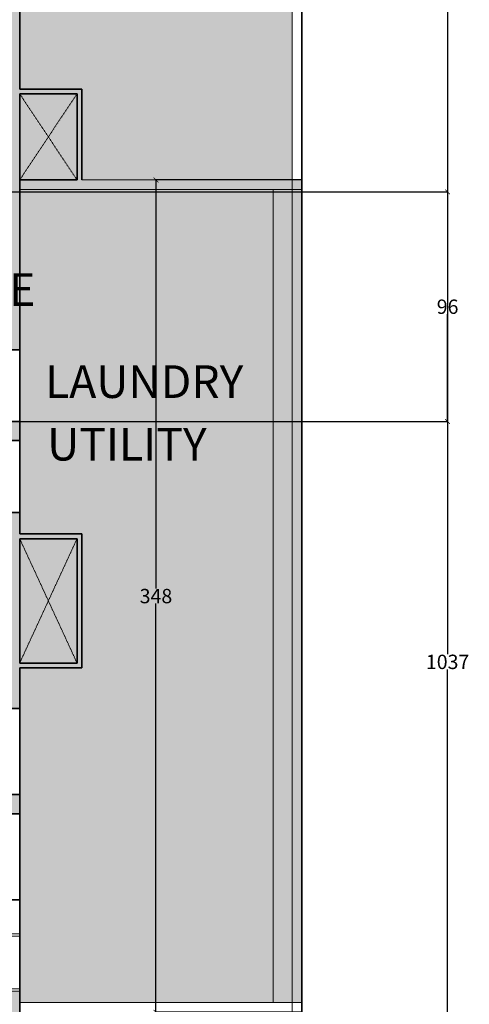
# Model space of a CAD drawing. Units: inches. Extents: x 1704 to 6393, y -157 to 1172.
# Tile 88 of 122: x 2605 to 2793, y 372 to 783. Entities that reach past the tile are written whole.
import ezdxf

# ---------------------------------------------------------------- set-up
doc = ezdxf.new("R2010")
doc.units = ezdxf.units.IN
doc.header["$MEASUREMENT"] = 0
doc.linetypes.add('HIDDEN', pattern=[0.375, 0.25, -0.125])
for name, color, linetype, lineweight in [('A-ANNO-DIMS', 7, 'Continuous', 13), ('A-AREA-IDEN', 7, 'Continuous', 18), ('A-FLOR-OPEN-HIDN', 8, 'HIDDEN', 13), ('A-WALL-PATT', 7, 'Continuous', 13), ('C-PROP', 7, 'Continuous', 35), ('L-HRDS', 8, 'Continuous', 18), ('L-PVMT-PATT', 8, 'Continuous', 13), ('WALLS', 7, 'Continuous', 35), ('WINDOWS', 2, 'Continuous', 18)]:
    doc.layers.add(name, color=color, linetype=linetype, lineweight=lineweight)
doc.layers.add('A-FLOR-PATT', color=7, linetype='Continuous', lineweight=13, true_color=0xf2f2f2)
doc.layers.add('L-HRDS-PATT', color=9, linetype='Continuous', lineweight=13, true_color=0xc5c1ba)
doc.styles.get("Standard").update_dxf_attribs({"font": 'arial.ttf'})
doc.dimstyles.get("Standard").update_dxf_attribs({"dimtxt": 6, "dimasz": 2, "dimexe": 0.18, "dimexo": 0.0625, "dimgap": 0.09, "dimtad": 0, "dimtih": 1, "dimtoh": 1, "dimdec": 1, "dimzin": 0, "dimdsep": 46, "dimlunit": 3, "dimtxsty": 'Standard', "dimblk": 'ARCHTICK', "dimcen": 0.09, "dimadec": 0, "dimazin": 0, "dimtfac": 1, "dimtdec": 1, "dimtofl": 0, "dimtmove": 0, "dimatfit": 3, "dimfxl": 1, "dimtolj": 1, "dimtzin": 0, "dimarcsym": 0})

# ---------------------------------------------------------------- blocks, each defined once
blk = doc.blocks.new('WIN-VENT-24')
for p, q in [((0, 0), (0, 24)), ((0, 24), (8, 24)), ((0, 23), (3.5, 23)), ((3.5, 23), (3.5, 1)), ((4.5, 23), (8, 23)), ((4.5, 23), (4.5, 1)), ((8, 24), (8, 0)), ((3.5, 1), (0, 1)), ((8, 1), (4.5, 1)), ((8, 0), (0, 0))]:
    blk.add_line(p, q)
blk = doc.blocks.new('_ArchTick')
at = {"color": 0, "linetype": 'ByBlock', "const_width": 0.15}
blk.add_lwpolyline([(-0.5, -0.5), (0.5, 0.5)], dxfattribs=at)
blk = doc.blocks.new('*D91')
at = {"layer": 'A-ANNO-DIMS', "color": 0, "lineweight": -2, "transparency": 16777216}
for p, q in [((2723.41, 1033.21), (2784.53, 1033.21)), ((2784.35, 1033.21), (2784.35, 517.87)), ((2784.35, -3.79), (2784.35, 511.56)), ((2723.41, -3.79), (2784.53, -3.79))]:
    blk.add_line(p, q, dxfattribs=at)
at = {"layer": 'Defpoints', "color": 0, "lineweight": -3, "transparency": 16777216}
for p in [(2723.35, 1033.21), (2784.35, 1033.21), (2723.35, -3.79)]:
    blk.add_point(p, dxfattribs=at)
at = {"layer": 'A-ANNO-DIMS', "color": 0, "lineweight": -2, "transparency": 16777216, "xscale": 2, "yscale": 2, "zscale": 2}
for p, rotation in [((2784.35, 1033.21), 90), ((2784.35, -3.79), 270)]:
    blk.add_blockref('_ArchTick', p, dxfattribs=dict(at, rotation=rotation))
at = {"layer": 'A-ANNO-DIMS', "color": 0, "transparency": 16777216, "insert": (2784.35, 514.71), "char_height": 6, "attachment_point": 5}
blk.add_mtext('\\A1;1037', dxfattribs=at)
blk = doc.blocks.new('*D97')
at = {"layer": 'A-ANNO-DIMS', "color": 0, "lineweight": -2, "transparency": 16777216}
for p, q in [((2723.29, 716.21), (2662.17, 716.21)), ((2662.35, 716.21), (2662.35, 545.37)), ((2662.35, 368.21), (2662.35, 539.06)), ((2723.29, 368.21), (2662.17, 368.21))]:
    blk.add_line(p, q, dxfattribs=at)
at = {"layer": 'Defpoints', "color": 0, "lineweight": -3, "transparency": 16777216}
for p in [(2662.35, 716.21), (2723.35, 716.21), (2723.35, 368.21)]:
    blk.add_point(p, dxfattribs=at)
at = {"layer": 'A-ANNO-DIMS', "color": 0, "lineweight": -2, "transparency": 16777216, "xscale": 2, "yscale": 2, "zscale": 2}
for p, rotation in [((2662.35, 716.21), 90), ((2662.35, 368.21), 270)]:
    blk.add_blockref('_ArchTick', p, dxfattribs=dict(at, rotation=rotation))
at = {"layer": 'A-ANNO-DIMS', "color": 0, "transparency": 16777216, "insert": (2662.35, 542.21), "char_height": 6, "attachment_point": 5}
blk.add_mtext('\\A1;348', dxfattribs=at)
blk = doc.blocks.new('*D101')
at = {"layer": 'A-ANNO-DIMS', "color": 0, "lineweight": -2, "transparency": 16777216}
for p, q in [((2547.41, 711.21), (2784.53, 711.21)), ((2784.35, 711.21), (2784.35, 666.37)), ((2784.35, 615.21), (2784.35, 660.06)), ((2547.41, 615.21), (2784.53, 615.21))]:
    blk.add_line(p, q, dxfattribs=at)
at = {"layer": 'Defpoints', "color": 0, "lineweight": -3, "transparency": 16777216}
for p in [(2547.35, 711.21), (2784.35, 711.21), (2547.35, 615.21)]:
    blk.add_point(p, dxfattribs=at)
at = {"layer": 'A-ANNO-DIMS', "color": 0, "lineweight": -2, "transparency": 16777216, "xscale": 2, "yscale": 2, "zscale": 2}
for p, rotation in [((2784.35, 711.21), 90), ((2784.35, 615.21), 270)]:
    blk.add_blockref('_ArchTick', p, dxfattribs=dict(at, rotation=rotation))
at = {"layer": 'A-ANNO-DIMS', "color": 0, "transparency": 16777216, "insert": (2784.35, 663.21), "char_height": 6, "attachment_point": 5}
blk.add_mtext('\\A1;96', dxfattribs=at)

msp = doc.modelspace()

# ---------------------------------------------------------------- hatches: boundary and pattern name
at = {"layer": 'A-FLOR-PATT'}
h = msp.add_hatch(color=256, dxfattribs=at)
h.dxf.hatch_style = 1
h.paths.add_polyline_path([(2629.349, 566.213), (2617.349, 540.213), (2629.349, 514.213)])
h.paths.add_polyline_path([(2629.349, 566.213), (2605.349, 566.213), (2617.349, 540.213)])
h.paths.add_polyline_path([(2605.349, 566.213), (2605.349, 514.213), (2617.349, 540.213)])
h.paths.add_polyline_path([(2617.349, 540.213), (2605.349, 514.213), (2629.349, 514.213)])
h.paths.add_polyline_path([(2617.349, 734.213), (2605.349, 716.213), (2629.349, 716.213)])
h.paths.add_polyline_path([(2629.349, 752.213), (2617.349, 734.213), (2629.349, 716.213)])
h.paths.add_polyline_path([(2617.349, 734.213), (2605.349, 752.213), (2605.349, 716.213)])
h.paths.add_polyline_path([(2629.349, 752.213), (2605.349, 752.213), (2617.349, 734.213)])
at = {"layer": 'A-WALL-PATT', "transparency": 33554643}
h = msp.add_hatch(color=256, dxfattribs=at)
h.dxf.hatch_style = 1
h.paths.add_polyline_path([(2167.349, 895.213), (2073.349, 895.213), (2073.349, 887.213), (2081.349, 887.213), (2167.349, 887.213)])
h.paths.add_polyline_path([(2465.349, 895.213), (2273.349, 895.213), (2273.349, 903.213), (2263.349, 903.213), (2263.349, 895.213), (2263.349, 887.213), (2325.349, 887.213), (2325.349, 863.213), (2333.349, 863.213), (2333.349, 887.213), (2465.349, 887.213)])
h.paths.add_polyline_path([(2533.349, 895.213), (2513.349, 895.213), (2513.349, 887.213), (2513.349, 861.213), (2517.349, 861.213), (2517.349, 887.213), (2533.349, 887.213)])
h.paths.add_polyline_path([(2605.349, 895.213), (2581.349, 895.213), (2581.349, 887.213), (2597.349, 887.213), (2597.349, 854.213), (2605.349, 854.213)])
h.paths.add_polyline_path([(2605.349, 752.213), (2629.349, 752.213), (2629.349, 716.213), (2605.349, 716.213), (2605.349, 712.213), (2719.349, 712.213), (2719.349, 716.213), (2631.349, 716.213), (2631.349, 754.213), (2605.349, 754.213), (2605.349, 794.213), (2597.349, 794.213), (2597.349, 787.213), (2517.349, 787.213), (2517.349, 813.213), (2513.349, 813.213), (2513.349, 783.213), (2517.349, 783.213), (2597.349, 783.213), (2597.349, 719.213), (2517.349, 719.213), (2517.349, 753.213), (2513.349, 753.213), (2513.349, 719.213), (2365.349, 719.213), (2365.349, 763.213), (2325.349, 763.213), (2325.349, 755.213), (2357.349, 755.213), (2357.349, 719.213), (2325.349, 719.213), (2325.349, 711.213), (2547.349, 711.213), (2547.349, 615.213), (2449.349, 615.213), (2449.349, 607.213), (2514.349, 607.213), (2514.349, 546.213), (2439.349, 546.213), (2425.349, 546.213), (2425.349, 607.213), (2425.349, 615.213), (2350.349, 615.213), (2350.349, 589.713), (2358.349, 589.713), (2358.349, 610.213), (2420.349, 610.213), (2420.349, 545.213), (2358.349, 545.213), (2358.349, 565.713), (2350.349, 565.713), (2350.349, 538.213), (2469.349, 538.213), (2469.349, 459.213), (2469.349, 372.213), (2423.349, 372.213), (2423.349, 364.213), (2473.349, 364.213), (2473.349, 318.213), (2477.349, 318.213), (2477.349, 364.213), (2547.349, 364.213), (2547.349, 352.213), (2549.349, 352.213), (2549.349, 364.213), (2597.349, 364.213), (2597.349, 328.213), (2549.349, 328.213), (2547.349, 328.213), (2547.349, 326.213), (2549.349, 326.213), (2597.349, 326.213), (2605.349, 326.213), (2605.349, 377.057), (2597.349, 377.057), (2597.349, 372.213), (2477.349, 372.213), (2477.349, 451.213), (2597.349, 451.213), (2605.349, 451.213), (2605.349, 459.213), (2597.349, 459.213), (2477.349, 459.213), (2477.349, 538.213), (2597.349, 538.213), (2597.349, 495.213), (2605.349, 495.213), (2605.349, 512.213), (2631.349, 512.213), (2631.349, 568.213), (2605.349, 568.213), (2605.349, 577.213), (2597.349, 577.213), (2597.349, 542.213), (2518.349, 542.213), (2518.349, 607.213), (2532.349, 607.213), (2605.349, 607.213), (2605.349, 615.213), (2597.349, 615.213), (2551.349, 615.213), (2551.349, 711.213), (2597.349, 711.213), (2597.349, 645.213), (2605.349, 645.213), (2605.349, 712.213), (2605.349, 716.213)])
h.paths.add_polyline_path([(2605.349, 566.213), (2629.349, 566.213), (2629.349, 514.213), (2605.349, 514.213)], flags=16)
h.paths.add_polyline_path([(2381.349, 372.213), (2349.349, 372.213), (2349.349, 202.213), (2337.349, 202.213), (2337.349, 194.213), (2349.349, 194.213), (2349.349, 90.213), (2349.349, 72.213), (2357.349, 72.213), (2357.349, 90.213), (2381.349, 90.213), (2381.349, 98.213), (2357.349, 98.213), (2357.349, 266.213), (2381.349, 266.213), (2381.349, 270.213), (2353.349, 270.213), (2353.349, 364.213), (2381.349, 364.213)])
h.paths.add_polyline_path([(2605.349, 302.213), (2597.349, 302.213), (2597.349, 270.213), (2477.349, 270.213), (2477.349, 294.213), (2473.349, 294.213), (2473.349, 270.213), (2423.349, 270.213), (2423.349, 266.213), (2597.349, 266.213), (2597.349, 218.213), (2605.349, 218.213)])
h.paths.add_polyline_path([(2605.349, 146.213), (2597.349, 146.213), (2597.349, 98.213), (2429.349, 98.213), (2429.349, 90.213), (2597.349, 90.213), (2597.349, 72.213), (2605.349, 72.213), (2605.349, 90.213)])
h.paths.add_polyline_path([(2225.349, 202.213), (2049.349, 202.213), (2049.349, 194.213), (2225.349, 194.213)])
h.paths.add_polyline_path([(2289.349, 202.213), (2277.349, 202.213), (2273.349, 202.213), (2269.516, 202.213), (2269.516, 194.213), (2273.349, 194.213), (2277.349, 194.213), (2289.349, 194.213)])
h.paths.add_polyline_path([(2273.349, 372.213), (2029.19, 372.213), (2029.19, 364.213), (2273.349, 364.213)])
h.paths.add_polyline_path([(2277.349, 545.213), (2213.349, 545.213), (2213.349, 573.213), (2205.349, 573.213), (2177.349, 573.213), (2177.349, 545.213), (2073.349, 545.213), (2073.349, 538.213), (2081.349, 538.213), (2277.349, 538.213)])
h.paths.add_polyline_path([(2181.349, 545.213), (2181.349, 569.213), (2205.349, 569.213), (2205.349, 545.213)], flags=16)
h.paths.add_polyline_path([(2277.349, 719.213), (2081.349, 719.213), (2073.349, 719.213), (2073.349, 711.213), (2154.575, 711.213), (2205.349, 711.213), (2205.349, 687.213), (2205.349, 629.213), (2213.349, 629.213), (2273.349, 629.213), (2273.349, 631.213), (2207.349, 631.213), (2207.349, 707.213), (2231.349, 707.213), (2231.349, 709.213), (2207.349, 709.213), (2207.349, 711.213), (2277.349, 711.213)])
at = {"layer": 'A-WALL-PATT', "transparency": 33554666}
h = msp.add_hatch(color=256, dxfattribs=at)
h.dxf.hatch_style = 1
h.paths.add_polyline_path([(2723.349, 712.213), (2719.349, 712.213), (2719.349, 372.213), (2723.349, 372.213)])
h.paths.add_polyline_path([(2723.349, 716.213), (2719.349, 716.213), (2719.349, 712.213), (2723.349, 712.213)])
at = {"layer": 'L-HRDS-PATT', "transparency": 33554661}
h = msp.add_hatch(color=256, dxfattribs=at)
h.dxf.hatch_style = 1
h.paths.add_polyline_path([(2719.349, 1033.213), (2664.349, 1033.213), (2664.349, 895.213), (2719.349, 895.213)])
h.paths.add_polyline_path([(2719.349, 895.213), (2664.349, 895.213), (2605.349, 895.213), (2605.349, 872.213), (2719.349, 872.213)])
h.paths.add_polyline_path([(2719.349, 872.213), (2605.349, 872.213), (2605.349, 854.213), (2601.349, 854.213, -0.1210664), (2618.034, 850.113), (2618.05, 850.14), (2619.349, 849.39), (2601.349, 818.213), (2605.349, 818.213), (2605.349, 794.213), (2605.349, 754.213), (2631.349, 754.213), (2631.349, 716.213), (2719.349, 716.213)])
at = {"layer": 'L-HRDS-PATT', "transparency": 33554666}
h = msp.add_hatch(color=256, dxfattribs=at)
h.dxf.hatch_style = 1
h.paths.add_polyline_path([(2711.349, 712.213), (2605.349, 712.213), (2605.349, 645.213), (2605.349, 615.213), (2605.349, 607.213), (2605.349, 577.213), (2605.349, 568.213), (2631.349, 568.213), (2631.349, 512.213), (2605.349, 512.213), (2605.349, 495.213), (2605.349, 459.213), (2605.349, 451.213), (2605.349, 415.213), (2605.349, 372.213), (2711.349, 372.213)])
at = {"layer": 'L-PVMT-PATT', "transparency": 33554528}
h = msp.add_hatch(dxfattribs=at)
h.set_pattern_fill('AR-CONC', color=256)
h.set_pattern_definition([(50, (0, 0), (7.172602, -0.627521), [0.75, -8.25]), (355, (0, 0), (-1.387513, 7.521921), [0.6, -6.6]), (100.45144, (0.598, -0.052), (5.785088, 6.8944), [0.637402, -7.011421]), (46.1842, (0, 2), (10.672413, -1.655193), [1.125, -12.375]), (96.63564, (0.889, 1.862), (9.34662, 9.741186), [0.956103, -10.517138]), (351.18416, (0, 2), (9.34662, 9.741186), [0.9, -9.9]), (21, (1, 1.5), (5.96907, -4.026189), [0.75, -8.25]), (326, (1, 1.5), (2.433153, 7.2515), [0.6, -6.6]), (71.45144, (1.4974, 1.1645), (8.402224, 3.225312), [0.637402, -7.011421]), (37.5, (0, 0), (0.1215986, 3.3289385), [0, -6.52, 0, -6.7, 0, -6.625]), (7.5, (0, 0), (2.6306954, 3.944117), [0, -3.82, 0, -6.37, 0, -2.525]), (327.5, (-2.23, 0), (5.3382244, -0.2255487), [0, -2.5, 0, -7.8, 0, -10.35]), (317.5, (-3.23, 0), (5.831862, 1.00105), [0, -3.25, 0, -5.18, 0, -7.35])])
h.paths.add_polyline_path([(2719.349, 712.213), (2711.349, 712.213), (2711.349, 372.213), (2719.349, 372.213)])

# ---------------------------------------------------------------- linework, layer by layer
at = {"layer": 'A-FLOR-OPEN-HIDN'}
for p, q in [((2605.349, 716.213), (2629.349, 752.213)), ((2605.349, 752.213), (2629.349, 716.213)), ((2605.349, 514.213), (2629.349, 566.213)), ((2605.349, 566.213), (2629.349, 514.213))]:
    msp.add_line(p, q, dxfattribs=at)
at = {"layer": 'C-PROP'}
msp.add_line((2723.349, -3.787), (2723.349, 1033.213), dxfattribs=at)
at = {"layer": 'L-HRDS'}
for p, q in [((2719.349, 5.658), (2719.349, 1033.213)), ((2631.349, 716.213), (2723.349, 716.213)), ((2605.349, 712.213), (2723.349, 712.213)), ((2711.349, 712.213), (2711.349, 372.213)), ((2605.349, 372.213), (2723.349, 372.213))]:
    msp.add_line(p, q, dxfattribs=at)
at = {"layer": 'WALLS'}
for p, q in [((2605.349, 754.213), (2605.349, 818.213)), ((2605.349, 754.213), (2631.349, 754.213)), ((2631.349, 754.213), (2631.349, 716.213)), ((2605.349, 716.213), (2605.349, 752.213)), ((2605.349, 752.213), (2629.349, 752.213)), ((2629.349, 752.213), (2629.349, 716.213)), ((2605.349, 716.213), (2629.349, 716.213)), ((2605.349, 712.213), (2605.349, 716.213)), ((2605.349, 645.213), (2605.349, 712.213)), ((2597.349, 645.213), (2605.349, 645.213)), ((2605.349, 645.213), (2605.349, 615.213)), ((2597.349, 615.213), (2605.349, 615.213)), ((2605.349, 607.213), (2605.349, 615.213)), ((2605.349, 607.213), (2532.349, 607.213)), ((2605.349, 607.213), (2605.349, 577.213)), ((2605.349, 577.213), (2597.349, 577.213)), ((2605.349, 568.213), (2605.349, 577.213)), ((2605.349, 568.213), (2631.349, 568.213)), ((2631.349, 568.213), (2631.349, 512.213)), ((2605.349, 566.213), (2629.349, 566.213)), ((2605.349, 514.213), (2605.349, 566.213)), ((2629.349, 566.213), (2629.349, 514.213)), ((2605.349, 514.213), (2629.349, 514.213)), ((2605.349, 512.213), (2631.349, 512.213)), ((2605.349, 495.213), (2605.349, 512.213)), ((2597.349, 495.213), (2605.349, 495.213)), ((2605.349, 495.213), (2605.349, 459.213)), ((2597.349, 459.213), (2605.349, 459.213)), ((2605.349, 451.213), (2605.349, 459.213)), ((2597.349, 451.213), (2605.349, 451.213)), ((2605.349, 451.213), (2605.349, 415.213)), ((2597.349, 415.213), (2605.349, 415.213)), ((2605.349, 218.213), (2605.349, 415.213))]:
    msp.add_line(p, q, dxfattribs=at)

# ---------------------------------------------------------------- block references
at = {"layer": 'WINDOWS'}
msp.add_blockref('WIN-VENT-24', (2597.349, 377.057), dxfattribs=at)

# ---------------------------------------------------------------- texts
at = {"layer": 'A-AREA-IDEN'}
for s, p in [('STORE', (2552.986, 663.555)), ('LAUNDRY', (2615.942, 625.045)), ('UTILITY', (2616.816, 598.878))]:
    msp.add_text(s, height=13.6672, dxfattribs=at).set_placement(p)

# ---------------------------------------------------------------- dimensions: what is measured, and where the dimension line sits
at = {"layer": 'A-ANNO-DIMS'}
for base, p1, p2, picture, middle in [((2784.349, 1033.213), (2723.349, -3.787), (2723.349, 1033.213), '*D91', (2784.349, 514.713)), ((2662.349, 716.213), (2723.349, 368.213), (2723.349, 716.213), '*D97', (2662.349, 542.213)), ((2784.349, 711.213), (2547.349, 615.213), (2547.349, 711.213), '*D101', (2784.349, 663.213))]:
    dim = msp.add_linear_dim(base=base, p1=p1, p2=p2, angle=90, dimstyle='Standard', override={"dimdec": 0, "dimlfac": 1, "dimrnd": 0, "dimzin": 0, "dimdsep": 46, "dimlunit": 2}, dxfattribs=at)
    dim.commit()
    dim.dimension.update_dxf_attribs({"geometry": picture, "text_midpoint": middle})

doc.saveas('drawing.dxf')
